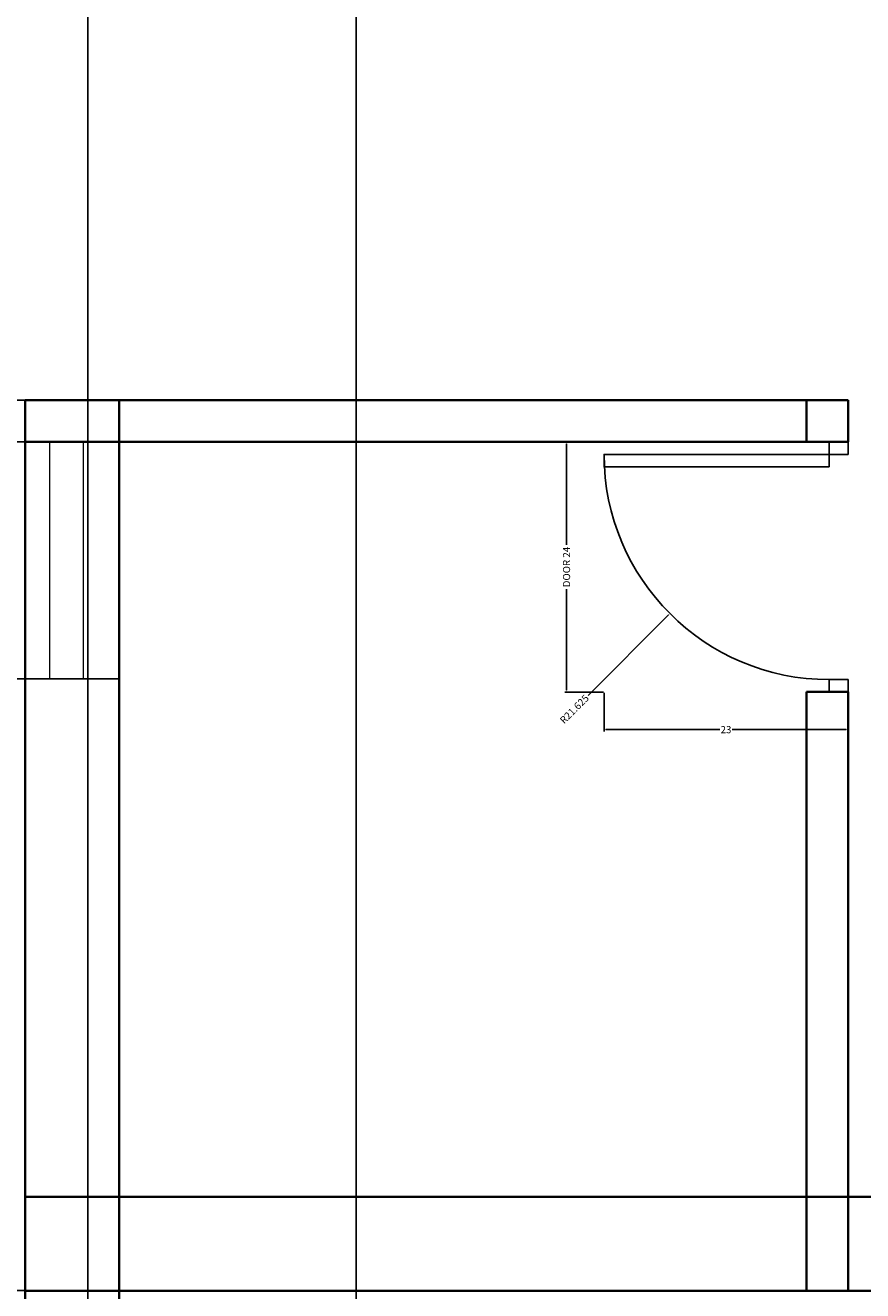
# Model space of a CAD drawing. Units: inches. Extents: x 867 to 1667, y -234 to 788.
# Tile 12 of 42: x 1071 to 1151, y 136 to 258. Entities that reach past the tile are written whole.
import ezdxf

# ---------------------------------------------------------------- set-up
doc = ezdxf.new("R2010")
doc.units = ezdxf.units.IN
doc.header["$MEASUREMENT"] = 0
for name, color, linetype, lineweight in [('A-ANNO-DIMS', 2, 'Continuous', 18), ('A-Door', 150, 'Continuous', 25), ('A-Glaz', 92, 'Continuous', 18), ('A-Wall', 7, 'Continuous', 35)]:
    doc.layers.add(name, color=color, linetype=linetype, lineweight=lineweight)
doc.layers.add('NET 01', color=8, linetype='Continuous')
doc.styles.get("Standard").update_dxf_attribs({"font": 'arial.ttf'})
doc.dimstyles.get("Standard").update_dxf_attribs({"dimtxt": 0.6875, "dimasz": 0.18, "dimexe": 0.18, "dimexo": 0.0625, "dimgap": 0.09, "dimtad": 0, "dimdec": 4, "dimzin": 0, "dimdsep": 46, "dimlunit": 4, "dimtxsty": 'Standard', "dimcen": 0.09, "dimadec": 0, "dimazin": 0, "dimtfac": 1, "dimtdec": 4, "dimtofl": 0, "dimtmove": 0, "dimatfit": 3, "dimfxl": 1, "dimtolj": 1, "dimtzin": 0, "dimarcsym": 0})

# ---------------------------------------------------------------- blocks, each defined once
blk = doc.blocks.new('A$C292B336C')
at = {"layer": 'A-Door'}
for points in [[(-0.05, 0), (-0.05, 0.9), (0, 0.9), (0, 0)], [(-0.95, 0), (-0.95, -0.075), (-0.9, -0.075), (-0.9, 0)], [(0, 0), (0, -0.075), (0.05, -0.075), (0.05, 0)]]:
    blk.add_lwpolyline(points, close=True, dxfattribs=at)
at = {"layer": 'NET 01'}
blk.add_arc((0, 0), 0.9, 90, 180, dxfattribs=at)
blk = doc.blocks.new('*D7')
at = {"layer": 'A-ANNO-DIMS', "color": 0, "lineweight": -2, "transparency": 16777216}
for p, q in [((1126.4, 217.62), (1122.68, 217.62)), ((1122.86, 217.44), (1122.86, 207.74)), ((1122.86, 193.77), (1122.86, 203.47)), ((1126.4, 193.59), (1122.68, 193.59))]:
    blk.add_line(p, q, dxfattribs=at)
at = {"layer": 'A-ANNO-DIMS', "color": 0, "transparency": 16777216}
for points in [[(1122.83, 217.44), (1122.89, 217.44), (1122.86, 217.62)], [(1122.83, 193.77), (1122.89, 193.77), (1122.86, 193.59)]]:
    blk.add_solid(points, dxfattribs=at)
at = {"layer": 'Defpoints', "color": 0, "transparency": 16777216}
for p in [(1122.86, 217.62), (1126.46, 217.62), (1126.46, 193.59)]:
    blk.add_point(p, dxfattribs=at)
at = {"layer": 'A-ANNO-DIMS', "color": 0, "transparency": 16777216, "insert": (1122.86, 205.6), "char_height": 0.6875, "attachment_point": 5, "rotation": 90}
blk.add_mtext('\\A1;DOOR 24', dxfattribs=at)
blk = doc.blocks.new('*D8')
at = {"layer": 'A-ANNO-DIMS', "color": 0, "lineweight": -2, "transparency": 16777216}
for p, q in [((1126.46, 193.53), (1126.46, 189.81)), ((1149.89, 193.53), (1149.89, 189.81)), ((1126.64, 189.99), (1137.58, 189.99)), ((1149.71, 189.99), (1138.76, 189.99))]:
    blk.add_line(p, q, dxfattribs=at)
at = {"layer": 'A-ANNO-DIMS', "color": 0, "transparency": 16777216}
for points in [[(1126.64, 190.02), (1126.64, 189.96), (1126.46, 189.99)], [(1149.71, 190.02), (1149.71, 189.96), (1149.89, 189.99)]]:
    blk.add_solid(points, dxfattribs=at)
at = {"layer": 'Defpoints', "color": 0, "transparency": 16777216}
for p in [(1126.46, 193.59), (1149.89, 193.59), (1126.46, 189.99)]:
    blk.add_point(p, dxfattribs=at)
at = {"layer": 'A-ANNO-DIMS', "color": 0, "transparency": 16777216, "insert": (1138.17, 189.99), "char_height": 0.688, "attachment_point": 5}
blk.add_mtext('\\A1;23', dxfattribs=at)
blk = doc.blocks.new('*D29')
at = {"layer": 'A-ANNO-DIMS', "color": 0, "lineweight": -2, "transparency": 16777216}
for p, q in [((1076.89, 623.55), (1076.89, -233.54)), ((1102.67, 623.55), (1102.67, -233.54)), ((1077.07, -233.36), (1088.52, -233.36)), ((1102.49, -233.36), (1091.03, -233.36))]:
    blk.add_line(p, q, dxfattribs=at)
at = {"layer": 'A-ANNO-DIMS', "color": 0, "transparency": 16777216}
for points in [[(1077.07, -233.33), (1077.07, -233.39), (1076.89, -233.36)], [(1102.49, -233.33), (1102.49, -233.39), (1102.67, -233.36)]]:
    blk.add_solid(points, dxfattribs=at)
at = {"layer": 'Defpoints', "color": 0, "transparency": 16777216}
for p in [(1076.89, 623.62), (1102.67, 623.62), (1102.67, -233.36)]:
    blk.add_point(p, dxfattribs=at)
at = {"layer": 'A-ANNO-DIMS', "color": 0, "transparency": 16777216, "insert": (1089.78, -233.36), "char_height": 0.688, "attachment_point": 5}
blk.add_mtext('\\A1;25.78', dxfattribs=at)
blk = doc.blocks.new('*D37')
at = {"layer": 'A-ANNO-DIMS', "color": 0, "lineweight": -2, "transparency": 16777216}
for p, q in [((1049.89, 257.55), (1049.89, -233.54)), ((1196.89, 257.55), (1196.89, -233.54)), ((1050.07, -233.36), (1122.57, -233.36)), ((1196.71, -233.36), (1124.2, -233.36))]:
    blk.add_line(p, q, dxfattribs=at)
at = {"layer": 'A-ANNO-DIMS', "color": 0, "transparency": 16777216}
for points in [[(1050.07, -233.33), (1050.07, -233.39), (1049.89, -233.36)], [(1196.71, -233.33), (1196.71, -233.39), (1196.89, -233.36)]]:
    blk.add_solid(points, dxfattribs=at)
at = {"layer": 'Defpoints', "color": 0, "transparency": 16777216}
for p in [(1049.89, 257.62), (1196.89, 257.62), (1196.89, -233.36)]:
    blk.add_point(p, dxfattribs=at)
at = {"layer": 'A-ANNO-DIMS', "color": 0, "transparency": 16777216, "insert": (1123.39, -233.36), "char_height": 0.688, "attachment_point": 5}
blk.add_mtext('\\A1;147', dxfattribs=at)
blk = doc.blocks.new('*D41')
at = {"layer": 'A-ANNO-DIMS', "color": 0, "lineweight": -2, "transparency": 16777216}
for p, q in [((1149.82, 221.62), (867.76, 221.62)), ((867.94, 221.44), (867.94, 179.85)), ((867.94, 136.3), (867.94, 177.88)), ((1149.82, 136.12), (867.76, 136.12))]:
    blk.add_line(p, q, dxfattribs=at)
at = {"layer": 'A-ANNO-DIMS', "color": 0, "transparency": 16777216}
for points in [[(867.91, 221.44), (867.97, 221.44), (867.94, 221.62)], [(867.91, 136.3), (867.97, 136.3), (867.94, 136.12)]]:
    blk.add_solid(points, dxfattribs=at)
at = {"layer": 'Defpoints', "color": 0, "transparency": 16777216}
for p in [(867.94, 221.62), (1149.89, 221.62), (1149.89, 136.12)]:
    blk.add_point(p, dxfattribs=at)
at = {"layer": 'A-ANNO-DIMS', "color": 0, "transparency": 16777216, "insert": (867.94, 178.87), "char_height": 0.688, "attachment_point": 5, "rotation": 90}
blk.add_mtext('\\A1;85.5', dxfattribs=at)
blk = doc.blocks.new('*D61')
at = {"layer": 'A-ANNO-DIMS', "color": 0, "lineweight": -2, "transparency": 16777216}
for p, q in [((1076.39, 217.62), (867.76, 217.62)), ((867.94, 217.44), (867.94, 207.78)), ((867.94, 195.06), (867.94, 204.72)), ((1079.82, 194.88), (867.76, 194.88))]:
    blk.add_line(p, q, dxfattribs=at)
at = {"layer": 'A-ANNO-DIMS', "color": 0, "transparency": 16777216}
for points in [[(867.91, 217.44), (867.97, 217.44), (867.94, 217.62)], [(867.91, 195.06), (867.97, 195.06), (867.94, 194.88)]]:
    blk.add_solid(points, dxfattribs=at)
at = {"layer": 'Defpoints', "color": 0, "transparency": 16777216}
for p in [(867.94, 217.62), (1076.46, 217.62), (1079.89, 194.88)]:
    blk.add_point(p, dxfattribs=at)
at = {"layer": 'A-ANNO-DIMS', "color": 0, "transparency": 16777216, "insert": (867.94, 206.25), "char_height": 0.688, "attachment_point": 5, "rotation": 90}
blk.add_mtext('\\A1;22.735', dxfattribs=at)
blk = doc.blocks.new('*D66')
at = {"layer": 'A-ANNO-DIMS', "color": 0, "lineweight": -2, "transparency": 16777216}
for p, q in [((1147.99, 216.42), (1148.17, 216.42)), ((1148.08, 216.33), (1148.08, 216.51)), ((1124.92, 193.26), (1132.66, 201))]:
    blk.add_line(p, q, dxfattribs=at)
at = {"layer": 'A-ANNO-DIMS', "color": 0, "transparency": 16777216}
blk.add_solid([(1132.64, 201.02), (1132.68, 200.98), (1132.79, 201.13)], dxfattribs=at)
at = {"layer": 'Defpoints', "color": 0, "transparency": 16777216}
for p in [(1148.08, 216.42), (1132.79, 201.13)]:
    blk.add_point(p, dxfattribs=at)
at = {"layer": 'A-ANNO-DIMS', "color": 0, "transparency": 16777216, "insert": (1123.61, 191.96), "char_height": 0.6875, "attachment_point": 5, "rotation": 44.9833}
blk.add_mtext('\\A1;R21.625', dxfattribs=at)

msp = doc.modelspace()

# ---------------------------------------------------------------- linework, layer by layer
at = {"layer": 'A-Glaz'}
for p, q in [((1073.2165, 217.617), (1073.2165, 194.8824)), ((1076.4575, 217.617), (1076.4575, 194.8824)), ((1070.8866, 194.8824), (1079.8866, 194.8824))]:
    msp.add_line(p, q, dxfattribs=at)
at = {"layer": 'A-Wall'}
for p, q in [((1070.8866, 221.617), (1070.8866, 136.117)), ((1149.8866, 221.617), (1070.8866, 221.617)), ((1070.8866, 221.617), (1070.8866, -55.9081)), ((1079.8866, 221.617), (1079.8866, 136.117)), ((1079.8866, 221.617), (1079.8866, -7.883)), ((1145.8866, 221.617), (1145.8866, 217.617)), ((1149.8866, 221.617), (1149.8866, 217.617)), ((1149.8866, 217.617), (1070.8866, 217.617)), ((1145.8866, 193.617), (1149.8866, 193.617)), ((1145.8866, 193.617), (1145.8866, 136.117)), ((1149.8866, 193.617), (1149.8866, 136.117)), ((1301.3542, 145.117), (1070.8866, 145.117)), ((1301.3542, 136.117), (1070.8866, 136.117))]:
    msp.add_line(p, q, dxfattribs=at)

# ---------------------------------------------------------------- block references
at = {"layer": 'A-Door', "xscale": 24.02746531046795, "yscale": 24.02746531046795, "zscale": 24.02746531046795, "rotation": 90}
msp.add_blockref('A$C292B336C', (1148.0846, 216.4157), dxfattribs=at)

# ---------------------------------------------------------------- dimensions: what is measured, and where the dimension line sits
at = {"layer": 'A-ANNO-DIMS'}
for base, p1, p2, override, picture, middle in [((1102.6661, -233.3581), (1076.8866, 623.617), (1102.6661, 623.617), {"dimdec": 2, "dimlfac": 1, "dimrnd": 0, "dimzin": 0, "dimdsep": 46, "dimlunit": 2}, '*D29', (1089.7763, -233.3581)), ((1196.8866, -233.3581), (1049.8866, 257.617), (1196.8866, 257.617), {"dimdec": 0, "dimlfac": 1, "dimrnd": 0, "dimzin": 0, "dimdsep": 46, "dimlunit": 2}, '*D37', (1123.3866, -233.3581))]:
    dim = msp.add_linear_dim(base=base, p1=p1, p2=p2, dimstyle='Standard', override=override, dxfattribs=at)
    dim.commit()
    dim.dimension.update_dxf_attribs({"geometry": picture, "text_midpoint": middle})
for base, p1, p2, angle, override, picture, middle in [((867.9366, 221.617), (1149.8866, 136.117), (1149.8866, 221.617), 90, {"dimdec": 1, "dimlfac": 1, "dimrnd": 0, "dimzin": 0, "dimdsep": 46, "dimlunit": 2}, '*D41', (867.9366, 178.867)), ((867.9366, 217.617), (1079.8866, 194.8824), (1076.4575, 217.617), 90, {"dimdec": 3, "dimlfac": 1, "dimrnd": 0, "dimzin": 0, "dimdsep": 46, "dimlunit": 2}, '*D61', (867.9366, 206.2497)), ((1126.4598, 189.9855), (1149.8866, 193.5896), (1126.4598, 193.5896), 180, {"dimdec": 0, "dimlfac": 1, "dimrnd": 0, "dimzin": 0, "dimdsep": 46, "dimlunit": 2}, '*D8', (1138.1732, 189.9855))]:
    dim = msp.add_linear_dim(base=base, p1=p1, p2=p2, angle=angle, dimstyle='Standard', override=override, dxfattribs=at)
    dim.commit()
    dim.dimension.update_dxf_attribs({"geometry": picture, "text_midpoint": middle})
dim = msp.add_linear_dim(base=(1122.8557, 217.617), p1=(1126.4598, 193.5896), p2=(1126.4598, 217.617), angle=90, text='DOOR <>', dimstyle='Standard', override={"dimdec": 0, "dimlfac": 1, "dimrnd": 0, "dimzin": 0, "dimdsep": 46, "dimlunit": 2}, dxfattribs=at)
dim.commit()
dim.dimension.update_dxf_attribs({"geometry": '*D7', "text_midpoint": (1122.8557, 205.6033)})
dim = msp.add_radius_dim(center=(1148.0846, 216.4157), mpoint=(1132.7891, 201.1291), dimstyle='Standard', override={"dimdec": 3, "dimlfac": 1, "dimrnd": 0, "dimzin": 0, "dimdsep": 46, "dimlunit": 2}, dxfattribs=at)
dim.commit()
dim.dimension.update_dxf_attribs({"geometry": '*D66', "text_midpoint": (1123.6119, 191.9572), "dimtype": 164})

doc.saveas('drawing.dxf')
